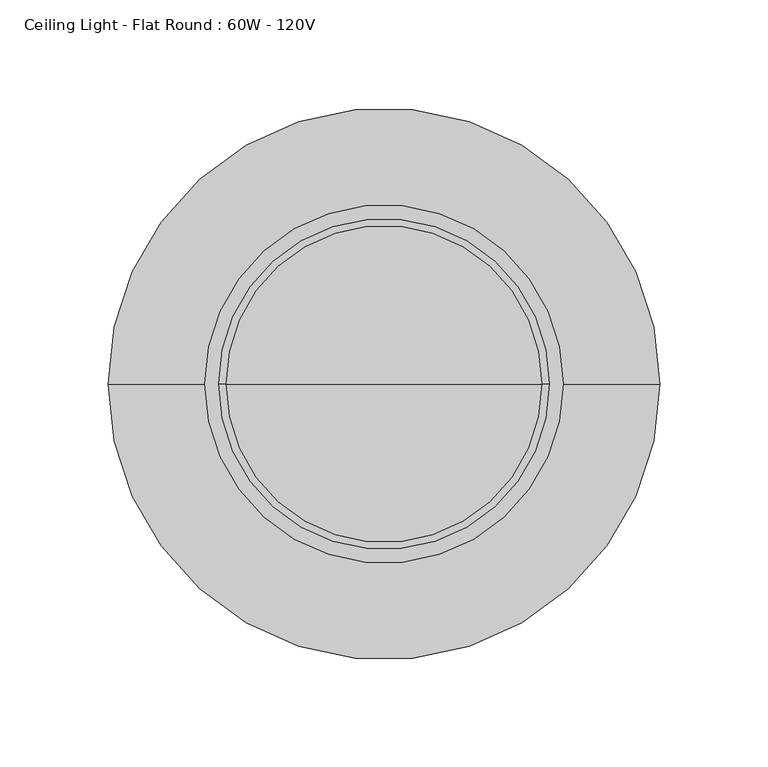
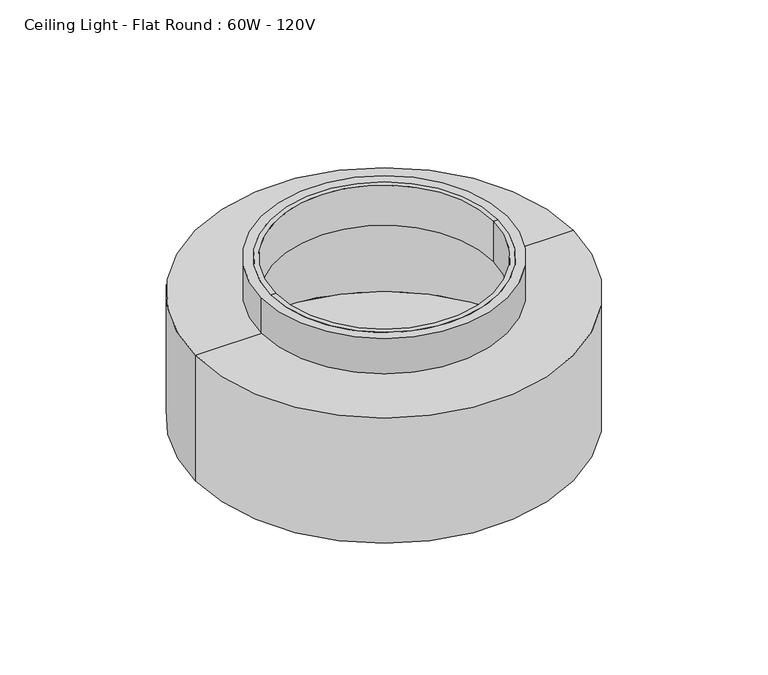
"""IFC4 building model written with IfcOpenShell, lengths in millimetres: light fixture geometry, Ceiling Light - Flat Round : 60W - 120V."""

from ifc_helpers import new_model, si_unit, point, frame, origin, origin_2d, place, context, project, spatial, polyline, circle_curve, trimmed, segment, composite_curve, outline, extrude, source, transform, mapped, element, save
from ifc_brep_helpers import plane_surface, cylinder_surface, revolved_surface, advanced_brep


def ceiling_light_flat_round_60w_120v_7c4c2a52(model_context):
    return source(origin(), model_context, "Body", "SolidModel", [
        advanced_brep(
        [(127.0, 0.0, 2413.0), (-127.0, 0.0, 2413.0), (-76.2, 0.0, 2413.0), (76.2, 0.0, 2413.0), (127.0, 0.0, 2324.1), (-127.0, 0.0, 2324.1), (0.0, 0.0, 2324.1), (123.825, 0.0, 2327.275), (-123.825, 0.0, 2327.275), (0.0, 0.0, 2327.275), (123.825, 0.0, 2409.825), (-123.825, 0.0, 2409.825), (73.025, 0.0, 2409.825), (-73.025, 0.0, 2409.825), (73.025, 0.0, 2438.4), (-73.025, 0.0, 2438.4), (76.2, 0.0, 2438.4), (-76.2, 0.0, 2438.4)],
        [
            (0, 1, circle_curve(frame((0.0, 0.0, 2413.0), z_axis=(0.0, 0.0, 1.0), x_axis=(-1.0, 0.0, 0.0)), 127.0)),
            (1, 2),
            (2, 3, circle_curve(frame((0.0, 0.0, 2413.0), z_axis=(0.0, 0.0, -1.0), x_axis=(-1.0, 0.0, 0.0)), 76.2)),
            (3, 0),
            (1, 0, circle_curve(frame((0.0, 0.0, 2413.0), z_axis=(0.0, 0.0, 1.0), x_axis=(-1.0, 0.0, 0.0)), 127.0)),
            (3, 2, circle_curve(frame((0.0, 0.0, 2413.0), z_axis=(0.0, 0.0, -1.0), x_axis=(-1.0, 0.0, 0.0)), 76.2)),
            (4, 5, circle_curve(frame((0.0, 0.0, 2324.1), z_axis=(0.0, 0.0, 1.0), x_axis=(-1.0, 0.0, 0.0)), 127.0)),
            (5, 1),
            (0, 4),
            (5, 4, circle_curve(frame((0.0, 0.0, 2324.1), z_axis=(0.0, 0.0, 1.0), x_axis=(-1.0, 0.0, 0.0)), 127.0)),
            (6, 5),
            (4, 6),
            (7, 8, circle_curve(frame((0.0, 0.0, 2327.275), z_axis=(0.0, 0.0, 1.0), x_axis=(-1.0, 0.0, 0.0)), 123.825)),
            (8, 9),
            (9, 7),
            (8, 7, circle_curve(frame((0.0, 0.0, 2327.275), z_axis=(0.0, 0.0, 1.0), x_axis=(-1.0, 0.0, 0.0)), 123.825)),
            (10, 11, circle_curve(frame((0.0, 0.0, 2409.825), z_axis=(0.0, 0.0, 1.0), x_axis=(-1.0, 0.0, 0.0)), 123.825)),
            (11, 8),
            (7, 10),
            (11, 10, circle_curve(frame((0.0, 0.0, 2409.825), z_axis=(0.0, 0.0, 1.0), x_axis=(-1.0, 0.0, 0.0)), 123.825)),
            (12, 13, circle_curve(frame((0.0, 0.0, 2409.825), z_axis=(0.0, 0.0, 1.0), x_axis=(-1.0, 0.0, 0.0)), 73.025)),
            (13, 11),
            (10, 12),
            (13, 12, circle_curve(frame((0.0, 0.0, 2409.825), z_axis=(0.0, 0.0, 1.0), x_axis=(-1.0, 0.0, 0.0)), 73.025)),
            (14, 15, circle_curve(frame((0.0, 0.0, 2438.4), z_axis=(0.0, 0.0, 1.0), x_axis=(-1.0, 0.0, 0.0)), 73.025)),
            (15, 13),
            (12, 14),
            (15, 14, circle_curve(frame((0.0, 0.0, 2438.4), z_axis=(0.0, 0.0, 1.0), x_axis=(-1.0, 0.0, 0.0)), 73.025)),
            (16, 17, circle_curve(frame((0.0, 0.0, 2438.4), z_axis=(0.0, 0.0, 1.0), x_axis=(-1.0, 0.0, 0.0)), 76.2)),
            (17, 15),
            (14, 16),
            (17, 16, circle_curve(frame((0.0, 0.0, 2438.4), z_axis=(0.0, 0.0, 1.0), x_axis=(-1.0, 0.0, 0.0)), 76.2)),
            (2, 17),
            (16, 3),
        ],
        [
            plane_surface(frame((0.0, 0.0, 2413.0), z_axis=(0.0, 0.0, 1.0), x_axis=(-1.0, 0.0, 0.0))),
            cylinder_surface(frame((0.0, 0.0, 2463.8), z_axis=(0.0, 0.0, -1.0), x_axis=(-1.0, 0.0, 0.0)), 127.0),
            plane_surface(frame((0.0, 0.0, 2324.1), z_axis=(0.0, 0.0, -1.0), x_axis=(-1.0, 0.0, 0.0))),
            plane_surface(frame((0.0, 0.0, 2327.275), z_axis=(0.0, 0.0, 1.0), x_axis=(-1.0, 0.0, 0.0))),
            revolved_surface(polyline([(-123.825, 0.0, 2327.275), (-123.825, 0.0, 2409.825)]), (0.0, 0.0, 2463.8), (0.0, 0.0, -1.0)),
            plane_surface(frame((0.0, 0.0, 2409.825), z_axis=(0.0, 0.0, -1.0), x_axis=(-1.0, 0.0, 0.0))),
            revolved_surface(polyline([(-73.025, 0.0, 2409.825), (-73.025, 0.0, 2438.4)]), (0.0, 0.0, 2463.8), (0.0, 0.0, -1.0)),
            plane_surface(frame((0.0, 0.0, 2438.4), z_axis=(0.0, 0.0, 1.0), x_axis=(-1.0, 0.0, 0.0))),
            cylinder_surface(frame((0.0, 0.0, 2463.8), z_axis=(0.0, 0.0, -1.0), x_axis=(-1.0, 0.0, 0.0)), 76.2),
        ],
        [
            (0, [[1, 2, 3, 4]]),
            (0, [[5, -4, 6, -2]]),
            (1, [[7, 8, -1, 9]]),
            (1, [[10, -9, -5, -8]]),
            (2, [[11, -7, 12]]),
            (2, [[-12, -10, -11]]),
            (3, [[13, 14, 15]]),
            (3, [[16, -15, -14]]),
            (4, [[17, 18, -13, 19]]),
            (4, [[20, -19, -16, -18]]),
            (5, [[21, 22, -17, 23]]),
            (5, [[24, -23, -20, -22]]),
            (6, [[25, 26, -21, 27]]),
            (6, [[28, -27, -24, -26]]),
            (7, [[29, 30, -25, 31]]),
            (7, [[32, -31, -28, -30]]),
            (8, [[-3, 33, -29, 34]]),
            (8, [[-6, -34, -32, -33]]),
        ],
    ),
        extrude(outline(composite_curve([segment(trimmed(circle_curve(origin_2d(), 82.55), [point((-82.55, 0.0))], [point((82.55, 0.0))], False, "CARTESIAN"), True, "CONTINUOUS"), segment(trimmed(circle_curve(origin_2d(), 82.55), [point((82.55, 0.0))], [point((-82.55, 0.0))], False, "CARTESIAN"), True, "CONTINUOUS")], self_intersect=False), holes=[composite_curve([segment(trimmed(circle_curve(origin_2d(), 76.2), [point((-76.2, 0.0))], [point((76.2, 0.0))], True, "CARTESIAN"), True, "CONTINUOUS"), segment(trimmed(circle_curve(origin_2d(), 76.2), [point((76.2, 0.0))], [point((-76.2, 0.0))], True, "CARTESIAN"), True, "CONTINUOUS")], self_intersect=False)]), frame((0.0, 0.0, 2413.0), z_axis=(0.0, 0.0, 1.0), x_axis=(1.0, 0.0, 0.0)), (0.0, 0.0, 1.0), 25.4),
    ])


if __name__ == "__main__":
    model = new_model("IFC4")
    model_context = context("Model", 3, world=origin())
    ifc_project = project(units=[si_unit("LENGTHUNIT", "METRE", prefix="MILLI")], contexts=[model_context])
    site = spatial("IfcSite", under=ifc_project)
    building = spatial("IfcBuilding", under=site)
    placement = place(None, origin())
    ceiling_light_flat_round_60w_120v_shape = ceiling_light_flat_round_60w_120v_7c4c2a52(model_context)
    element("IfcLightFixture", 1, ObjectType="Ceiling Light - Flat Round : 60W - 120V", at=placement, inside=building, context=model_context, shape_type="MappedRepresentation", body=[
        mapped(ceiling_light_flat_round_60w_120v_shape, transform((0.0, 0.0, 0.0), x_axis=(1.0, 0.0, 0.0), y_axis=(0.0, 1.0, 0.0), z_axis=(0.0, 0.0, 1.0))),
    ])
    save(model, "model.ifc")

# Revit data of these elements
# Type "Ceiling Light - Flat Round : 60W - 120V"
#   Lamp = "A-19"
#   Assembly Code = "D5020220"
#   Wattage = 60 W
#   built-in parameter 1150110 = 1 (stored number, unit not read)
#   built-in parameter 1114217 = 1 (stored number, unit not read)
#   built-in parameter 1150109 = 1 (stored number, unit not read)
#   built-in parameter 1150113 = 1 (stored number, unit not read)
#   built-in parameter 1150115 = 1 (stored number, unit not read)
#   built-in parameter 1150105 = 272.155 (stored number, unit not read)
#   Light Source Symbol Size = 2' - 0"
#   built-in parameter 1150112 = 1 (stored number, unit not read)
#   built-in parameter 1150114 = 1 (stored number, unit not read)
#   built-in parameter 1150107 = 2800 (stored number, unit not read)
#   built-in parameter 1150106 = 2.72155 (stored number, unit not read)
#   Emit from Circle Diameter = 0' - 10"
#   built-in parameter 1150104 = 1.32387 (stored number, unit not read)
#   Ballast Voltage = 120 V
#   built-in parameter 1114218 = 1 (stored number, unit not read)
#   built-in parameter 1150133 = 10 (stored number, unit not read)
#   Lumens = 855 lm
#   Apparent Load = 60 VA
#   built-in parameter 1150134 = 4
#   built-in parameter 1150137 = 1
#   Color Filter = 16777215
#   built-in parameter 1140040 [instance default] = 1
#   Ballast Number of Poles = 1
#   Light Box Material = Steel, Paint Finish, Dark Gray, Matte
#   Diffuser Material = Glass, White, High Luminance
#   Wattage Comments = ""
#   Emit Shape Visible in Rendering = no
#   Dimming Lamp Color Temperature Shift = (empty or 0)
#   Default Elevation = 0
# Element 1 (IfcLightFixture, "Ceiling Light - Flat Round : 60W - 120V")
#   Materials on its faces: "Glass, White, High Luminance", "Steel, Paint Finish, Dark Gray, Matte"
# Materials
#   "Steel, Paint Finish, Dark Gray, Matte": class "Metal", colour RGB 98 98 98, transparency 0, Description = "Steel, paint finish, dark gray, matte", Cost = 0
#   "Glass, White, High Luminance": class "Glass", colour RGB 120 120 120, transparency 0, Description = "physical material", Cost = 0
